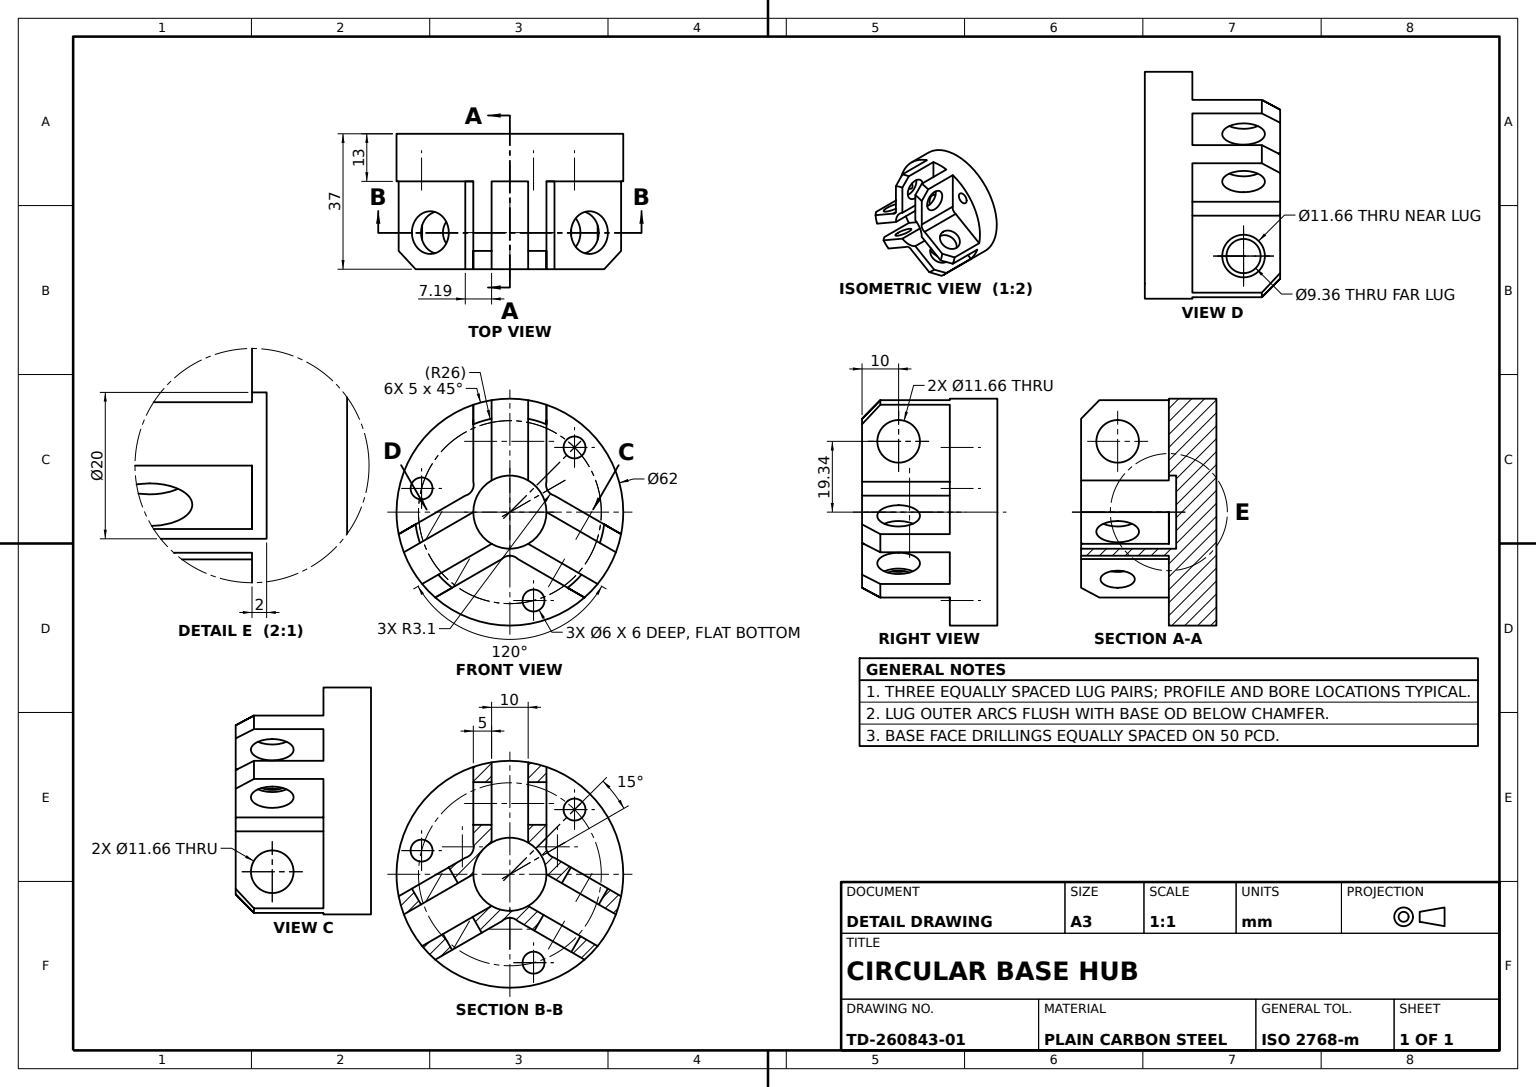
SolidWorks part; units mm, degrees
material "Plain Carbon Steel"
ref_plane "Front Plane" through (0, 0, 0) normal (0, 0, 1) x (1, 0, 0)
ref_plane "Top Plane" through (0, 0, 0) normal (0, 1, 0) x (1, 0, 0)
ref_plane "Right Plane" through (0, 0, 0) normal (1, 0, 0) x (0, 0, -1)
sketch "Base Disc Sketch" plane through (0, 0, 0) normal (0, 0, 1) x (1, 0, 0)
  circle A0 centre (0, 0) radius 31
  dimension "D1" = 62
extrude "Base Disc" add sketch "Base Disc Sketch" along normal blind 13
sketch "Base Slot Sketch 3x" plane through (0, 0, 0) normal (0, 0, 1) x (1, 0, 0)
  line L0 (0, 0) -> (0, -25) construction
  line L2 (-6.4705, -24.1481) -> (0, 0) construction
  circle A0 centre (0, 0) radius 25 construction
  circle A1 centre (-6.4705, -24.1481) radius 3
  circle A2 centre (-17.6777, 17.6777) radius 3
  circle A3 centre (24.1481, 6.4705) radius 3
  point P12 (0, 0)
  dimension "D1" = 15
  dimension "D2" = 3
  dimension "D3" = 6
  dimension "D6" = 50
extrude "Base Slots 3x" cut sketch "Base Slot Sketch 3x" along normal blind 6
sketch "Clamp Lug Sketch" plane through (0, 0, 0) normal (0, 0, 1) x (1, 0, 0)
  line L2 (5, 8.6603) -> (5, 30.5941)
  line L4 (10, 8.3066) -> (10, 29.3428)
  line L8 (12.1937, 4.5069) -> (30.4116, -6.0111)
  line L10 (10, 0) -> (10, 30.5941) construction
  line L12 (5, 0) -> (5, 30.5941) construction
  line L13 (10, 0) -> (28.9953, -10.9669)
  arc A5 (28.9953, -10.9669) -> (30.4116, -6.0111) centre (0, 0) ccw
  arc A6 (10, 29.3428) -> (5, 30.5941) centre (0, 0) ccw
  arc A9 (12.1937, 4.5069) -> (10, 8.3066) centre (12.9967, 7.5037) cw
  arc A11 (10, 0) -> (5, 8.6603) centre (0, 0) ccw
  point P8 (5, 31)
  point P9 (-5, 0)
  point P10 (-5, 31)
  point P12 (-5, 30.5941)
  point P16 (-10, 0)
  point P17 (-10, 30.5941)
  point P41 (0, 0)
  point P48 (0, 0)
  dimension "D5" = 7.1937
  dimension "D1" = 31
  dimension "D2" = 3.1024
  dimension "D4" = 10
  dimension "D3" = 5
extrude "Clamp Lug" add sketch "Clamp Lug Sketch" against normal blind 24
sketch "Lug Hole A Sketch" plane through (10, 0, 0) normal (1, 0, 0) x (0, 0, -1)
  line L0 (24, 8.3066) -> (24, 29.3428) construction
  line L1 (24, 29.3428) -> (0, 29.3428) construction
  circle A0 centre (14, 19.3428) radius 4.6801
  dimension "D3" = 9.3602
  dimension "D1" = 10
  dimension "D2" = 10
extrude "Lug Hole A" cut sketch "Lug Hole A Sketch" against normal through all
sketch "Lug Hole B Sketch" plane through (5, 8.6603, 0) normal (0.5, 0.866, 0) x (0.866, -0.5, 0)
  line L0 (29.3428, 24) -> (29.3428, 0) construction
  line L1 (29.3428, 24) -> (8.3066, 24) construction
  circle A0 centre (19.3428, 14) radius 5.8304
  dimension "D3" = 11.6608
  dimension "D1" = 10
  dimension "D2" = 10
extrude "Lug Hole B" cut sketch "Lug Hole B Sketch" against normal through all
pattern_circular "Clamp Lug Pattern 3x" count 3 over 360 about axis through (0, 0, 0) along (0, 0, 1) of "Clamp Lug", "Lug Hole A", "Lug Hole B"
sketch "Face Recess Sketch" plane through (0, 0, 0) normal (0, 0, -1) x (-1, 0, 0)
  circle A0 centre (0, 0) radius 10
  dimension "D1" = 20
extrude "Face Recess 2mm" cut sketch "Face Recess Sketch" against normal blind 2
chamfer "Lug Chamfer 5mm" distance 5 angle 45 6 edges at (7.5261, 30.0726, -24) (29.8066, -8.5185, -24) (-29.8066, -8.5185, -24) (-7.5261, 30.0726, -24) (22.2806, -21.554, -24) (-22.2806, -21.554, -24)
